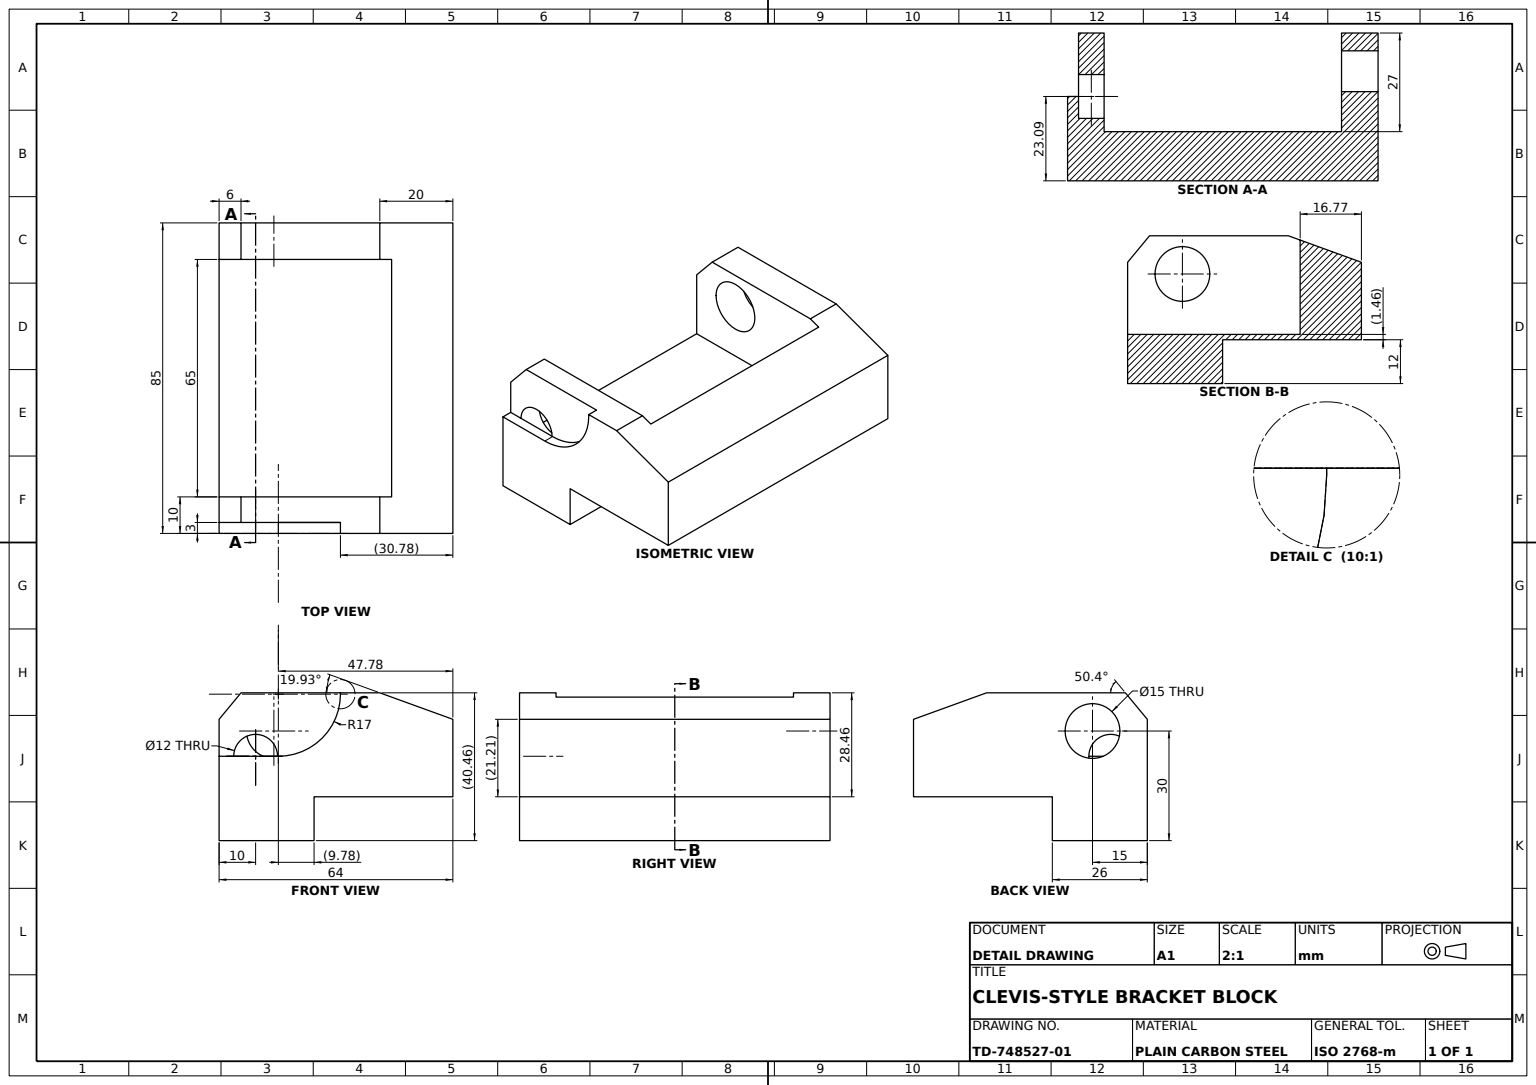
SolidWorks part; units mm, degrees
material "Plain Carbon Steel"
ref_plane "Front Plane" through (0, 0, 0) normal (0, 0, 1) x (1, 0, 0)
ref_plane "Top Plane" through (0, 0, 0) normal (0, 1, 0) x (1, 0, 0)
ref_plane "Right Plane" through (0, 0, 0) normal (1, 0, 0) x (0, 0, -1)
sketch "Bearing Block Profile" plane through (0, 0, 0) normal (1, 0, 0) x (0, 0, -1)
  line L0 (0, 0) -> (38, 0)
  line L1 (38, 0) -> (38, -12)
  line L2 (38, -12) -> (64, -12)
  line L3 (64, -12) -> (64, 21.2067)
  line L6 (20, 28.4587) -> (0, 21.2067)
  line L7 (0, 21.2067) -> (0, 0)
  line L8 (64, 21.2067) -> (58, 28.4587)
  line L9 (58, 28.4587) -> (20, 28.4587)
  dimension "D1" = 64
  dimension "D2" = 20
  dimension "D3" = 12
  dimension "D4" = 26
  dimension "D5" = 6
  dimension "D6" = 21.2067
  dimension "D7" = 28.4587
extrude "Bearing Block" add sketch "Bearing Block Profile" along normal mid plane 85
sketch "Lug Slot Profile" plane through (0, 28.4587, 0) normal (0, 1, 0) x (1, 0, 0)
  line L0 (0, 64) -> (0, 0) construction
  line L1 (42.5, 64) -> (-42.5, 64) construction
  line L3 (-32.5, 16.7684) -> (32.5, 16.7684)
  line L4 (-32.5, 16.7684) -> (-32.5, 66.7684)
  line L5 (-32.5, 66.7684) -> (32.5, 66.7684)
  line L6 (32.5, 16.7684) -> (32.5, 66.7684)
  line L7 (42.5, 20) -> (-42.5, 20) construction
  point P9 (0, 16.7684)
  dimension "D1" = 65
  dimension "D2" = 50
  dimension "D3" = 46.7684
extrude "Lug Slot 65x50" cut sketch "Lug Slot Profile" against normal blind 27 contours L4 L5 L6 L3
sketch "Bore Ø15 Sketch" plane through (42.5, 0, 0) normal (1, 0, 0) x (0, 0, -1)
  line L0 (64, -12) -> (64, 21.2067) construction
  line L1 (38, -12) -> (64, -12) construction
  circle A0 centre (49, 18) radius 7.5
  dimension "D3" = 15
  dimension "D1" = 15
  dimension "D2" = 30
extrude "Pivot Bore Ø15" cut sketch "Bore Ø15 Sketch" against normal up to surface (10 mm away) up to face at (32.5, 18.0547, -39.9228)
sketch "Lug Recess A Profile" plane through (-42.5, 0, 0) normal (-1, 0, 0) x (0, 0, 1)
  line L0 (-58, 28.4587) -> (-20, 28.4587) construction
  line L2 (-64, -12) -> (-64, 21.2067) construction
  line L3 (-63.5518, 21.7484) -> (-58, 28.4587)
  line L4 (-64, 21.2067) -> (-58, 28.4587) construction
  line L5 (-58, 28.4587) -> (-30.7834, 28.4587)
  arc A0 (-30.7834, 28.4587) -> (-64, 23.0028) centre (-47.7794, 28.0912) cw
  line M3 (-20, 28.4587) -> (-58, 28.4587)
  line M4 (-58, 28.4587) -> (-64, 21.2067)
  dimension "D1" = 17
  dimension "D2" = 30.7834
  dimension "D3" = 47.7794
extrude "Lug Recess A 3mm" cut sketch "Lug Recess A Profile" against normal blind 3 contours A0 M3 M4
sketch "Lug Recess B Profile" plane through (-42.5, 0, 0) normal (-1, 0, 0) x (0, 0, 1)
  line L0 (-47.7794, 11.0912) -> (-64, 11.0912)
  line L1 (-64, -12) -> (-64, 21.2067) construction
  line L2 (-64, 11.0912) -> (-64, 21.2067)
  line L3 (-64, 21.2067) -> (-63.5518, 21.7484)
  line L4 (-63.5518, 21.7484) -> (-47.7794, 11.0912)
  line L5 (-38, 0) -> (-38, -12) construction
  arc A0 (-63.5518, 21.7484) -> (-30.7834, 28.4587) centre (-47.7794, 28.0912) ccw construction
  arc A1 (-63.5518, 21.7484) -> (-30.7834, 28.4587) centre (-47.7794, 28.0912) ccw construction
  dimension "D1" = 9.7794
extrude "Lug Recess B 3mm" cut sketch "Lug Recess B Profile" against normal blind 3
sketch "Bore Ø10 Sketch" plane through (-39.5, 0, 0) normal (-1, 0, 0) x (0, 0, 1)
  line L0 (-64, 11.0912) -> (-47.7794, 11.0912) construction
  line L1 (-64, 21.2067) -> (-64, 11.0912) construction
  circle A0 centre (-54, 11.0912) radius 6
  dimension "D2" = 12
  dimension "D1" = 10
extrude "Pivot Bore Ø10" cut sketch "Bore Ø10 Sketch" against normal up to surface (7 mm away) contours A0 up to face at (-32.5, 18.0547, -39.9228)
